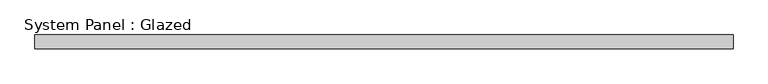
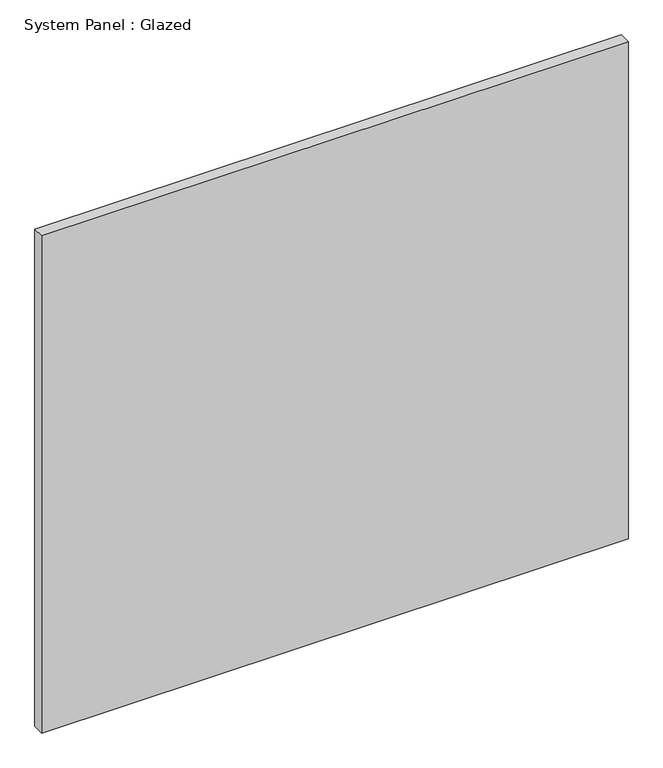
"""IFC4 building model written with IfcOpenShell, lengths in millimetres: plate geometry, System Panel : Glazed."""

from ifc_helpers import new_model, si_unit, origin, origin_with_axes, place, context, project, spatial, polyline, outline, extrude, source, transform, mapped, element, save


def system_panel_glazed_2adfbad0(model_context):
    return source(origin(), model_context, "Body", "SweptSolid", [
        extrude(outline(polyline([(645.3496911, 19.05), (-645.3496911, 19.05), (-645.3496911, 44.45), (645.3496911, 44.45), (645.3496911, 19.05)])), origin_with_axes(), (0.0, 0.0, 1.0), 1155.7),
    ])


if __name__ == "__main__":
    model = new_model("IFC4")
    model_context = context("Model", 3, world=origin())
    ifc_project = project(units=[si_unit("LENGTHUNIT", "METRE", prefix="MILLI")], contexts=[model_context])
    site = spatial("IfcSite", under=ifc_project)
    building = spatial("IfcBuilding", under=site)
    placement = place(None, origin())
    system_panel_glazed_shape = system_panel_glazed_2adfbad0(model_context)
    element("IfcPlate", 1, ObjectType="System Panel : Glazed", at=placement, inside=building, context=model_context, shape_type="MappedRepresentation", body=[
        mapped(system_panel_glazed_shape, transform((0.0, 0.0, 0.0), x_axis=(1.0, 0.0, 0.0), y_axis=(0.0, 1.0, 0.0), z_axis=(0.0, 0.0, 1.0))),
    ])
    save(model, "model.ifc")

# Revit data of these elements
# Type "System Panel : Glazed"
#   Construction Type Id = "GSP4R"
#   Analytic Construction = "1/8 in Pilkington single glazing"
#   Visual Light Transmittance = 0.9
#   Solar Heat Gain Coefficient = 0.86
#   Heat Transfer Coefficient (U) = 1.18115 BTU/(h·ft²·°F)
# Element 1 (IfcPlate, "System Panel : Glazed")
#   Materials on its faces: "Glass"
# Materials
#   "Glass": class "Glass", colour RGB 0 128 192, transparency 0.75, Description = "Soda Lime Glass", Cost = 0
